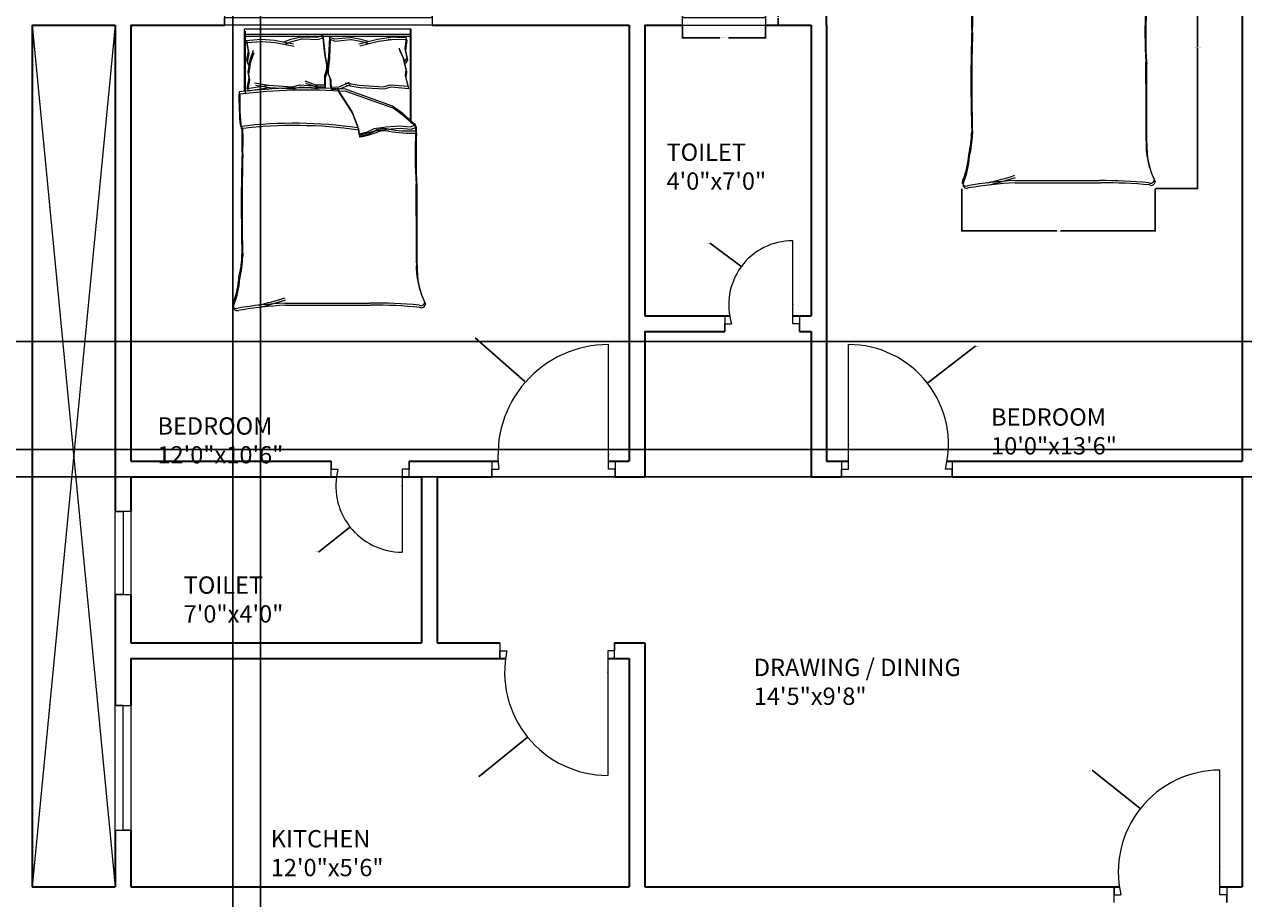
# Model space of a CAD drawing. Units: inches. Extents: x 1937 to 2996, y 1402 to 2323.
# Tile 7 of 10: x 2290 to 2643, y 1944 to 2197. Entities that reach past the tile are written whole.
import ezdxf

# ---------------------------------------------------------------- set-up
doc = ezdxf.new("R2010")
doc.units = ezdxf.units.IN
for name, color, linetype, lineweight in [('A-ANNO-DIMS', 2, 'Continuous', 18), ('A-AREA-IDEN', 7, 'Continuous', 18), ('A-DOOR', 11, 'Continuous', 18), ('A-FLOR-OPEN', 81, 'Continuous', 18), ('A-FURN', 8, 'Continuous', 13), ('A-GLAZ', 141, 'Continuous', 18), ('A-WALL', 7, 'Continuous', 35)]:
    doc.layers.add(name, color=color, linetype=linetype, lineweight=lineweight)
doc.styles.get("Standard").update_dxf_attribs({"font": 'arial.ttf'})
doc.dimstyles.get("Standard").update_dxf_attribs({"dimtxt": 0.18, "dimasz": 0.18, "dimexe": 0.18, "dimexo": 0.0625, "dimgap": 0.09, "dimtad": 0, "dimtih": 1, "dimtoh": 1, "dimdec": 4, "dimzin": 0, "dimdsep": 46, "dimtxsty": 'Standard', "dimcen": 0.09, "dimadec": 0, "dimazin": 0, "dimtfac": 1, "dimtdec": 4, "dimtofl": 0, "dimtmove": 0, "dimatfit": 3, "dimfxl": 1, "dimtolj": 1, "dimtzin": 0, "dimarcsym": 0})

# ---------------------------------------------------------------- blocks, each defined once
blk = doc.blocks.new('BED-DOUBLE')
for p, q in [((-24.01, -18.11), (-24.01, 0)), ((-24.01, -18.11), (-24.01, 0)), ((-24.01, 0), (24.01, 0)), ((23.78, 0), (23.78, -26.61)), ((23.78, 0), (23.78, -26.61)), ((24.01, 0), (24.01, -0.64)), ((-24.01, -1.53), (23.78, -1.53)), ((-24.01, -1.53), (23.78, -1.53)), ((-23.78, -18.75), (-23.78, -0.64)), ((-23.78, -18.75), (-23.78, -0.64)), ((-23.78, -2.17), (24.01, -2.17)), ((-23.78, -2.17), (24.01, -2.17)), ((-23.59, -3.34), (-19.3, -3.01)), ((-23.59, -3.34), (-19.31, -3.01)), ((-23.59, -3.32), (-23.01, -6.5)), ((-23.59, -3.32), (-23.01, -6.5)), ((-19.31, -3.01), (-19.2, -3.03)), ((-19.3, -3.01), (-19.2, -3.03)), ((-19.2, -3.03), (-15.38, -3.32)), ((-19.2, -3.03), (-15.38, -3.32)), ((-15.38, -3.32), (-9.88, -4.33)), ((-15.38, -3.32), (-9.88, -4.33)), ((-12.63, -3.75), (-10.61, -3.03)), ((-12.63, -3.75), (-10.61, -3.03)), ((-10.61, -3.03), (-7.71, -2.3)), ((-10.61, -3.03), (-7.71, -2.3)), ((-10.38, -3.67), (-7.49, -2.94)), ((-10.38, -3.67), (-7.49, -2.94)), ((-7.71, -2.3), (-7.39, -2.3)), ((-7.71, -2.3), (-7.39, -2.3)), ((-7.49, -2.94), (-7.16, -2.94)), ((-7.49, -2.94), (-7.16, -2.94)), ((-7.39, -2.3), (-2.95, -2.45)), ((-7.39, -2.3), (-2.95, -2.45)), ((-7.16, -2.94), (-2.72, -3.09)), ((-7.16, -2.94), (-2.72, -3.09)), ((-2.95, -2.45), (-1.5, -1.87)), ((-2.95, -2.45), (-1.5, -1.87)), ((-2.72, -3.09), (-1.27, -2.51)), ((-2.72, -3.09), (-1.27, -2.51)), ((-1.5, -1.87), (-0.92, -7.22)), ((-1.5, -1.87), (-0.92, -7.22)), ((-1.27, -2.51), (-0.7, -7.86)), ((-1.27, -2.51), (-0.7, -7.86)), ((0.49, -2.49), (0.25, -7.87)), ((0.49, -2.49), (0.25, -7.87)), ((0.72, -3.13), (0.48, -8.51)), ((0.72, -3.13), (0.48, -8.51)), ((1.97, -2.98), (0.49, -2.49)), ((1.97, -2.98), (0.49, -2.49)), ((2.2, -3.62), (0.72, -3.13)), ((2.2, -3.62), (0.72, -3.13)), ((6.4, -2.56), (1.97, -2.98)), ((6.4, -2.56), (1.97, -2.98)), ((6.63, -3.2), (2.2, -3.62)), ((6.63, -3.2), (2.2, -3.62)), ((6.72, -2.54), (6.4, -2.56)), ((6.72, -2.54), (6.4, -2.56)), ((6.95, -3.18), (6.63, -3.2)), ((6.95, -3.18), (6.63, -3.2)), ((9.65, -3.08), (6.72, -2.54)), ((9.65, -3.08), (6.72, -2.54)), ((9.88, -3.72), (6.95, -3.18)), ((9.88, -3.72), (6.95, -3.18)), ((14.43, -3.07), (9.01, -4.42)), ((14.43, -3.07), (9.01, -4.42)), ((11.72, -3.67), (9.65, -3.08)), ((11.72, -3.67), (9.65, -3.08)), ((18.23, -2.54), (14.43, -3.07)), ((18.23, -2.54), (14.43, -3.07)), ((18.46, -3.18), (14.66, -3.71)), ((18.46, -3.18), (14.66, -3.71)), ((22.63, -2.56), (17.23, -2.46)), ((17.23, -2.46), (18.23, -2.54)), ((22.63, -2.56), (17.23, -2.46)), ((17.23, -2.46), (18.23, -2.54)), ((22.86, -3.2), (17.45, -3.1)), ((17.45, -3.1), (18.46, -3.18)), ((22.86, -3.2), (17.45, -3.1)), ((17.45, -3.1), (18.46, -3.18)), ((22.63, -2.56), (22.25, -5.77)), ((22.63, -2.56), (22.25, -5.77)), ((22.86, -3.2), (22.48, -6.41)), ((22.86, -3.2), (22.48, -6.41)), ((24.01, -0.64), (24.01, -27.25)), ((24.01, -0.64), (24.01, -27.25)), ((-23.01, -6.5), (-23.45, -9.1)), ((-23.01, -6.5), (-23.45, -9.1)), ((-23.36, -3.98), (-19.08, -3.65)), ((-23.36, -3.98), (-19.08, -3.65)), ((-23.36, -3.96), (-22.78, -7.14)), ((-23.36, -3.96), (-22.78, -7.14)), ((-22.43, -8.96), (-21.42, -6.21)), ((-22.43, -8.96), (-21.42, -6.21)), ((-22.21, -9.59), (-21.19, -6.85)), ((-22.2, -9.59), (-21.19, -6.85)), ((-19.08, -3.65), (-18.97, -3.67)), ((-19.08, -3.65), (-18.97, -3.67)), ((-18.97, -3.67), (-15.15, -3.96)), ((-18.97, -3.67), (-15.15, -3.96)), ((-15.15, -3.96), (-9.65, -4.97)), ((-15.15, -3.96), (-9.65, -4.97)), ((-12.4, -4.39), (-10.38, -3.67)), ((-12.4, -4.39), (-10.38, -3.67)), ((14.66, -3.71), (9.24, -5.06)), ((14.66, -3.71), (9.24, -5.06)), ((11.94, -4.31), (9.88, -3.72)), ((11.94, -4.31), (9.88, -3.72)), ((21.83, -8.26), (20.64, -5.58)), ((21.82, -8.26), (20.64, -5.58)), ((22.05, -8.9), (20.87, -6.22)), ((22.05, -8.9), (20.87, -6.22)), ((22.25, -5.77), (22.84, -8.34)), ((22.25, -5.77), (22.84, -8.34)), ((22.48, -6.41), (23.07, -8.98)), ((22.48, -6.41), (23.07, -8.98)), ((-23.45, -9.1), (-22.87, -10.11)), ((-23.45, -9.1), (-22.87, -10.11)), ((-22.78, -7.14), (-23.22, -9.74)), ((-22.78, -7.14), (-23.22, -9.74)), ((-23.22, -9.74), (-22.64, -10.75)), ((-23.22, -9.74), (-22.64, -10.75)), ((-23.01, -12.57), (-22.43, -8.96)), ((-23.01, -12.57), (-22.43, -8.96)), ((-22.78, -13.21), (-22.2, -9.59)), ((-22.78, -13.21), (-22.21, -9.59)), ((-0.92, -7.22), (-0.35, -10.4)), ((-0.92, -7.22), (-0.35, -10.4)), ((-0.7, -7.86), (-0.12, -11.04)), ((-0.7, -7.86), (-0.12, -11.04)), ((-0.35, -10.4), (-0.35, -11.7)), ((-0.35, -10.4), (-0.35, -11.7)), ((0.25, -7.87), (-0.13, -11.08)), ((0.25, -7.87), (-0.13, -11.08)), ((0.48, -8.51), (0.1, -11.72)), ((0.48, -8.51), (0.1, -11.72)), ((22.63, -11.83), (21.82, -8.26)), ((22.63, -11.83), (21.83, -8.26)), ((22.86, -12.47), (22.05, -8.9)), ((22.86, -12.47), (22.05, -8.9)), ((22.84, -8.34), (22.33, -9.38)), ((22.84, -8.34), (22.33, -9.38)), ((23.07, -8.98), (22.56, -10.02)), ((23.07, -8.98), (22.56, -10.02)), ((-22.72, -14.16), (-23.01, -12.57)), ((-22.72, -14.16), (-23.01, -12.57)), ((-22.49, -14.8), (-22.78, -13.21)), ((-22.49, -14.8), (-22.78, -13.21)), ((-0.35, -11.7), (-0.92, -13.58)), ((-0.35, -11.7), (-0.92, -13.58)), ((-0.92, -13.58), (-0.92, -16.26)), ((-0.92, -13.58), (-0.92, -16.26)), ((-0.12, -12.34), (-0.7, -14.22)), ((-0.12, -12.34), (-0.7, -14.22)), ((-0.13, -11.08), (-0.05, -12.38)), ((-0.13, -11.08), (-0.05, -12.38)), ((-0.12, -11.04), (-0.12, -12.34)), ((-0.12, -11.04), (-0.12, -12.34)), ((-0.05, -12.38), (0.65, -14.22)), ((-0.05, -12.38), (0.65, -14.22)), ((0.1, -11.72), (0.18, -13.02)), ((0.1, -11.72), (0.18, -13.02)), ((0.18, -13.02), (0.87, -14.86)), ((0.18, -13.02), (0.87, -14.86)), ((22.44, -13.43), (22.63, -11.83)), ((22.44, -13.43), (22.63, -11.83)), ((23.21, -16.57), (22.44, -13.43)), ((23.21, -16.57), (22.44, -13.43)), ((22.67, -14.07), (22.86, -12.47)), ((22.67, -14.07), (22.86, -12.47)), ((23.44, -17.21), (22.67, -14.07)), ((23.44, -17.21), (22.67, -14.07)), ((-23.3, -17.34), (-22.72, -14.16)), ((-23.3, -17.34), (-22.72, -14.16)), ((-18.2, -16.62), (-23.3, -17.34)), ((-18.2, -16.62), (-23.3, -17.34)), ((-23.07, -17.98), (-22.49, -14.8)), ((-23.07, -17.98), (-22.49, -14.8)), ((-17.98, -17.26), (-23.07, -17.98)), ((-17.98, -17.26), (-23.07, -17.98)), ((-21.1, -15.63), (-17.07, -16.3)), ((-21.1, -15.63), (-17.07, -16.3)), ((-20.87, -16.27), (-16.84, -16.93)), ((-20.87, -16.27), (-16.84, -16.93)), ((-17.07, -16.3), (-18.2, -16.62)), ((-17.07, -16.3), (-18.2, -16.62)), ((-16.84, -16.93), (-17.98, -17.26)), ((-16.84, -16.93), (-17.98, -17.26)), ((-17.07, -16.3), (-10.06, -16.73)), ((-17.07, -16.3), (-10.06, -16.73)), ((-16.84, -16.93), (-9.83, -17.37)), ((-16.84, -16.93), (-9.83, -17.37)), ((-10.06, -16.73), (-8.1, -16.17)), ((-10.06, -16.73), (-8.1, -16.17)), ((-9.83, -17.37), (-7.87, -16.81)), ((-9.83, -17.37), (-7.87, -16.81)), ((-8.1, -16.17), (-2.97, -16.57)), ((-8.1, -16.17), (-2.97, -16.57)), ((-7.87, -16.81), (-2.74, -17.21)), ((-7.87, -16.81), (-2.74, -17.21)), ((-3.38, -16.26), (-6.53, -15.17)), ((-3.38, -16.26), (-6.53, -15.17)), ((-3.15, -16.9), (-6.3, -15.81)), ((-3.15, -16.9), (-6.3, -15.81)), ((-0.92, -16.26), (-3.38, -16.26)), ((-0.92, -16.26), (-3.38, -16.26)), ((-0.7, -16.9), (-3.15, -16.9)), ((-0.7, -16.9), (-3.15, -16.9)), ((-0.7, -14.22), (-0.7, -16.9)), ((-0.7, -14.22), (-0.7, -16.9)), ((0.65, -14.22), (0.81, -16.89)), ((0.65, -14.22), (0.81, -16.89)), ((0.81, -16.89), (3.27, -16.74)), ((0.81, -16.89), (3.27, -16.74)), ((0.87, -14.86), (1.04, -17.53)), ((0.87, -14.86), (1.04, -17.53)), ((1.04, -17.53), (3.49, -17.38)), ((1.04, -17.53), (3.49, -17.38)), ((2.77, -17.38), (6.97, -23.88)), ((2.77, -17.38), (6.96, -23.88)), ((3.27, -16.74), (6.34, -15.45)), ((3.27, -16.74), (6.34, -15.45)), ((3.49, -17.38), (6.56, -16.09)), ((3.49, -17.38), (6.56, -16.09)), ((13.16, -20.32), (4.82, -17.38)), ((13.16, -20.32), (4.82, -17.38)), ((5.08, -15.63), (9.11, -16.3)), ((5.08, -15.63), (9.11, -16.3)), ((5.31, -16.27), (9.34, -16.93)), ((5.31, -16.27), (9.34, -16.93)), ((9.11, -16.3), (16.12, -16.73)), ((9.11, -16.3), (16.12, -16.73)), ((9.34, -16.93), (16.35, -17.37)), ((9.34, -16.93), (16.35, -17.37)), ((16.12, -16.73), (18.08, -16.17)), ((16.12, -16.73), (18.08, -16.17)), ((16.35, -17.37), (18.31, -16.81)), ((16.35, -17.37), (18.31, -16.81)), ((18.08, -16.17), (23.21, -16.57)), ((18.08, -16.17), (23.21, -16.57)), ((18.31, -16.81), (23.44, -17.21)), ((18.31, -16.81), (23.44, -17.21)), ((3, -18.02), (7.19, -24.52)), ((3, -18.02), (7.19, -24.52)), ((13.39, -20.96), (5.05, -18.02)), ((13.39, -20.96), (5.05, -18.02)), ((18.74, -22.33), (13.16, -20.32)), ((18.74, -22.33), (13.16, -20.32)), ((18.96, -22.97), (13.39, -20.96)), ((18.96, -22.97), (13.39, -20.96)), ((6.96, -23.88), (8.67, -28.37)), ((6.97, -23.88), (8.67, -28.37)), ((7.19, -24.52), (8.9, -29)), ((7.19, -24.52), (8.9, -29)), ((21.68, -24.5), (18.74, -22.33)), ((21.68, -24.5), (18.74, -22.33)), ((21.91, -25.13), (18.96, -22.97)), ((21.91, -25.13), (18.96, -22.97)), ((25.38, -27.75), (21.68, -24.5)), ((25.38, -27.75), (21.68, -24.5)), ((16.88, -28.37), (20.75, -28.06)), ((16.88, -28.37), (20.75, -28.06)), ((20.75, -28.06), (23.85, -28.37)), ((20.75, -28.06), (23.85, -28.37)), ((25.61, -28.39), (21.91, -25.13)), ((25.61, -28.39), (21.91, -25.13)), ((23.85, -28.37), (25.38, -27.75)), ((23.85, -28.37), (25.38, -27.75)), ((25.46, -29.49), (25.38, -27.75, 3.87)), ((25.46, -29.49), (25.38, -27.75, 3.87)), ((8.67, -28.37), (8.98, -30.38)), ((8.67, -28.37), (8.98, -30.38)), ((8.9, -29), (9.21, -31.02)), ((8.9, -29), (9.21, -31.02)), ((8.98, -30.38), (11.46, -29.76)), ((8.98, -30.38), (11.46, -29.76)), ((9.21, -31.02), (11.68, -30.4)), ((9.21, -31.02), (11.68, -30.4)), ((11.46, -29.76), (13.47, -28.83)), ((11.46, -29.76), (13.47, -28.83)), ((11.68, -30.4), (13.7, -29.47)), ((11.68, -30.4), (13.7, -29.47)), ((13.47, -28.83), (16.88, -28.37)), ((13.47, -28.83), (16.88, -28.37)), ((13.7, -29.47), (17.11, -29)), ((13.7, -29.47), (17.1, -29)), ((17.1, -29), (20.98, -28.69)), ((17.11, -29), (20.98, -28.69)), ((20.98, -28.69), (24.07, -29)), ((20.98, -28.69), (24.07, -29)), ((24.07, -29), (25.61, -28.39)), ((24.07, -29), (25.61, -28.39)), ((25.69, -30.13), (25.61, -28.39, 3.87)), ((25.69, -30.13), (25.61, -28.39, 3.87)), ((-12.42, -79.25), (12.19, -79.25)), ((-12.42, -79.25), (12.19, -79.25)), ((-12.19, -79.88), (12.42, -79.88)), ((-12.19, -79.88), (12.42, -79.88))]:
    blk.add_line(p, q)
for centre, radius, start, end in [((-6.13, -182.05), 164.97, 86.0865, 96.7821), ((-6.13, -182.05), 164.97, 86.0865, 96.7821), ((57.68, -20.1), 83.31, 178.7218, 185.604), ((57.68, -20.1), 83.31, 178.7218, 185.604), ((57.91, -20.74), 83.31, 178.7218, 185.604), ((57.91, -20.74), 83.31, 178.7218, 185.604), ((-5.9, -182.69), 164.97, 86.0865, 96.7821), ((-5.9, -182.69), 164.97, 86.0865, 96.7821), ((-9.73, -156.32), 129.02, 81.7845, 96.9006), ((-9.73, -156.32), 129.02, 81.7845, 96.9006), ((-9.5, -156.96), 129.02, 81.7845, 96.9006), ((-9.5, -156.96), 129.02, 81.7845, 96.9006), ((-194.79, -31.17), 170.11, 358.4762, 1.0082), ((-194.79, -31.17), 170.11, 358.4762, 1.0082), ((-194.56, -31.81), 170.11, 358.4762, 1.0082), ((-194.56, -31.81), 170.11, 358.4762, 1.0082), ((9.15, -30.44), 0.185, 160.2464, 271.1377), ((9.15, -30.44), 0.185, 160.2464, 271.1377), ((3.67, -1.48), 29.65, 280.6617, 289.8806), ((3.67, -1.48), 29.65, 280.6617, 289.8806), ((9.38, -31.08), 0.185, 160.2464, 271.1377), ((9.38, -31.08), 0.185, 160.2464, 271.1377), ((3.9, -2.12), 29.65, 280.6617, 289.8806), ((3.9, -2.12), 29.65, 280.6617, 289.8806), ((16.26, -35.07), 6.22, 78.6608, 113.7384), ((16.26, -35.07), 6.22, 78.6608, 113.7384), ((16.49, -35.71), 6.22, 78.6608, 113.7384), ((16.49, -35.71), 6.22, 78.6608, 113.7384), ((23.84, 6.66), 36.18, 259.8763, 272.5657), ((23.84, 6.66), 36.18, 259.8763, 272.5657), ((24.07, 6.02), 36.18, 259.8763, 272.5657), ((24.07, 6.02), 36.18, 259.8763, 272.5657), ((154.78, -36.32), 129.5, 176.9791, 183.8365), ((154.78, -36.32), 129.5, 176.9791, 183.8365), ((155.01, -36.95), 129.5, 176.9791, 183.8365), ((155.01, -36.95), 129.5, 176.9791, 183.8365), ((457.34, -50.61), 482.31, 178.2277, 181.7185), ((457.34, -50.61), 482.31, 178.2277, 181.7185), ((457.57, -51.25), 482.31, 178.2277, 181.7185), ((457.57, -51.25), 482.31, 178.2277, 181.7185), ((-4536.23, -67.82), 4561.86, 0.00217, 0.28689), ((-4536.23, -67.82), 4561.86, 0.00217, 0.28689), ((-4536, -68.46), 4561.86, 0.00217, 0.28689), ((-4536, -68.46), 4561.86, 0.00217, 0.28689), ((-54.38, -64.52), 29.63, 346.0648, 358.9113), ((-54.38, -64.52), 29.63, 346.0648, 358.9113), ((-54.16, -65.15), 29.63, 346.0648, 358.9113), ((-54.16, -65.15), 29.63, 346.0648, 358.9113), ((48.67, -68.67), 23.07, 177.4714, 206.4681), ((48.67, -68.67), 23.07, 177.4714, 206.4681), ((48.9, -69.31), 23.07, 177.4714, 206.4681), ((48.9, -69.31), 23.07, 177.4714, 206.4681), ((-49.14, -70.28), 23.56, 337.9751, 356.652), ((-49.14, -70.28), 23.56, 337.9751, 356.652), ((-48.92, -70.91), 23.56, 337.9751, 356.652), ((-48.92, -70.91), 23.56, 337.9751, 356.652), ((-26.4, -79.72), 1.09, 146.1736, 293.4781), ((-26.4, -79.72), 1.09, 146.1736, 293.4781), ((-26.17, -80.36), 1.09, 146.1736, 293.4781), ((-26.17, -80.36), 1.09, 146.1736, 293.4781), ((-6.06, -200.84), 121.76, 92.9958, 99.4091), ((-6.06, -200.84), 121.76, 92.9958, 99.4091), ((-5.83, -201.48), 121.76, 92.9958, 99.4091), ((-5.83, -201.48), 121.76, 92.9958, 99.4091), ((-44.71, 23.71), 106.46, 283.3832, 287.7053), ((-44.71, 23.71), 106.46, 283.3832, 287.7053), ((-44.48, 23.07), 106.46, 283.3832, 287.7053), ((-44.48, 23.07), 106.46, 283.3832, 287.7053), ((13.67, -212.28), 133.04, 84.4998, 90.6351), ((13.67, -212.28), 133.04, 84.4998, 90.6351), ((13.9, -212.92), 133.04, 84.4998, 90.6351), ((13.9, -212.92), 133.04, 84.4998, 90.6351), ((26.93, -78.87), 1.1, 242.6588, 356.02), ((26.93, -78.87), 1.1, 242.6588, 356.02), ((27.15, -79.51), 1.1, 242.6588, 356.02), ((27.15, -79.51), 1.1, 242.6588, 356.02)]:
    blk.add_arc(centre, radius, start, end)
blk = doc.blocks.new('WINDOW-60IN')
for p, q in [((0, 2.25), (0, -2.25)), ((0, 2.25), (60, 2.25)), ((0, -2.25), (0, 0)), ((0, 0), (60, 0)), ((60, 0), (60, 2.25)), ((60, 2.25), (60, -2.25)), ((60, -2.25), (0, -2.25))]:
    blk.add_line(p, q)
blk = doc.blocks.new('WINDOW-36IN')
for p, q in [((0, 2.25), (0, -2.25)), ((0, 2.25), (36, 2.25)), ((36, 0), (36, 2.25)), ((36, 2.25), (36, -2.25)), ((0, -2.25), (0, 0)), ((0, 0), (36, 0)), ((36, -2.25), (0, -2.25))]:
    blk.add_line(p, q)
blk = doc.blocks.new('WINDOW-24IN-JAMB-B')
for p, q in [((0, -2.25), (0, 2.25)), ((0, 2.25), (0, 0)), ((24, 2.25), (0, 2.25)), ((0, 0), (24, 0)), ((24, 0), (24, 2.25)), ((24, 2.25), (24, -2.25)), ((0, -2.25), (24, -2.25))]:
    blk.add_line(p, q)
blk = doc.blocks.new('VOID-MARK-24X249')
for p, q in [((24, 249), (0, 0)), ((0, 249), (24, 0))]:
    blk.add_line(p, q)
blk = doc.blocks.new('*D9')
at = {"layer": 'A-ANNO-DIMS', "color": 0, "lineweight": -2, "transparency": 16777216}
for p, q in [((2617.12, 2230.66), (2629.47, 2230.66)), ((2629.29, 2230.48), (2629.29, 2190.07)), ((2629.29, 2149.29), (2629.29, 2189.7)), ((2617.12, 2149.11), (2629.47, 2149.11))]:
    blk.add_line(p, q, dxfattribs=at)
at = {"layer": 'A-ANNO-DIMS', "color": 0, "transparency": 16777216}
for points in [[(2629.26, 2230.48), (2629.32, 2230.48), (2629.29, 2230.66)], [(2629.26, 2149.29), (2629.32, 2149.29), (2629.29, 2149.11)]]:
    blk.add_solid(points, dxfattribs=at)
at = {"layer": 'Defpoints', "color": 0, "transparency": 16777216}
for p in [(2617.06, 2230.66), (2629.29, 2230.66), (2617.06, 2149.11)]:
    blk.add_point(p, dxfattribs=at)
at = {"layer": 'A-ANNO-DIMS', "color": 0, "transparency": 16777216, "insert": (2629.29, 2189.88), "char_height": 0.18, "attachment_point": 5}
blk.add_mtext('\\A1;DOUBLE BED 82 TYP.', dxfattribs=at)
blk = doc.blocks.new('*D10')
at = {"layer": 'A-ANNO-DIMS', "color": 0, "lineweight": -2, "transparency": 16777216}
for p, q in [((2561.23, 2149.05), (2561.23, 2136.7)), ((2617.06, 2149.05), (2617.06, 2136.7)), ((2561.41, 2136.88), (2588.62, 2136.88)), ((2616.88, 2136.88), (2589.67, 2136.88))]:
    blk.add_line(p, q, dxfattribs=at)
at = {"layer": 'A-ANNO-DIMS', "color": 0, "transparency": 16777216}
for points in [[(2561.41, 2136.91), (2561.41, 2136.85), (2561.23, 2136.88)], [(2616.88, 2136.91), (2616.88, 2136.85), (2617.06, 2136.88)]]:
    blk.add_solid(points, dxfattribs=at)
at = {"layer": 'Defpoints', "color": 0, "transparency": 16777216}
for p in [(2561.23, 2149.11), (2617.06, 2149.11), (2617.06, 2136.88)]:
    blk.add_point(p, dxfattribs=at)
at = {"layer": 'A-ANNO-DIMS', "color": 0, "transparency": 16777216, "insert": (2589.14, 2136.88), "char_height": 0.18, "attachment_point": 5}
blk.add_mtext('\\A1;56 TYP.', dxfattribs=at)
blk = doc.blocks.new('*D17')
at = {"layer": 'A-ANNO-DIMS', "color": 0, "lineweight": -2, "transparency": 16777216}
for p, q in [((2480.52, 2196.24), (2480.52, 2192.53)), ((2504.52, 2196.24), (2504.52, 2192.53)), ((2480.7, 2192.71), (2491.28, 2192.71)), ((2504.34, 2192.71), (2493.75, 2192.71))]:
    blk.add_line(p, q, dxfattribs=at)
at = {"layer": 'A-ANNO-DIMS', "color": 0, "transparency": 16777216}
for points in [[(2480.7, 2192.74), (2480.7, 2192.68), (2480.52, 2192.71)], [(2504.34, 2192.74), (2504.34, 2192.68), (2504.52, 2192.71)]]:
    blk.add_solid(points, dxfattribs=at)
at = {"layer": 'Defpoints', "color": 0, "transparency": 16777216}
for p in [(2480.52, 2196.31), (2504.52, 2196.31), (2504.52, 2192.71)]:
    blk.add_point(p, dxfattribs=at)
at = {"layer": 'A-ANNO-DIMS', "color": 0, "transparency": 16777216, "insert": (2492.52, 2192.71), "char_height": 0.18, "attachment_point": 5}
blk.add_mtext('\\A1;WINDOW B 24 TYP.', dxfattribs=at)
blk = doc.blocks.new('*D18')
at = {"layer": 'A-ANNO-DIMS', "color": 0, "lineweight": -2, "transparency": 16777216}
for p, q in [((2504.58, 2200.81), (2508.3, 2200.81)), ((2508.12, 2200.63), (2508.12, 2198.74)), ((2508.12, 2196.49), (2508.12, 2198.37)), ((2504.58, 2196.31), (2508.3, 2196.31))]:
    blk.add_line(p, q, dxfattribs=at)
at = {"layer": 'A-ANNO-DIMS', "color": 0, "transparency": 16777216}
for points in [[(2508.09, 2200.63), (2508.15, 2200.63), (2508.12, 2200.81)], [(2508.09, 2196.49), (2508.15, 2196.49), (2508.12, 2196.31)]]:
    blk.add_solid(points, dxfattribs=at)
at = {"layer": 'Defpoints', "color": 0, "transparency": 16777216}
for p in [(2504.52, 2200.81), (2508.12, 2200.81), (2504.52, 2196.31)]:
    blk.add_point(p, dxfattribs=at)
at = {"layer": 'A-ANNO-DIMS', "color": 0, "transparency": 16777216, "insert": (2508.12, 2198.56), "char_height": 0.18, "attachment_point": 5}
blk.add_mtext('\\A1;5 TYP.', dxfattribs=at)
blk = doc.blocks.new('*D36')
at = {"layer": 'A-ANNO-DIMS', "color": 0, "lineweight": -2, "transparency": 16777216}
for p, q in [((2350.61, 1896.12), (2350.61, 2283.14)), ((2350.79, 2282.96), (2354.46, 2282.96)), ((2358.43, 2282.96), (2354.76, 2282.96)), ((2358.61, 1896.12), (2358.61, 2283.14))]:
    blk.add_line(p, q, dxfattribs=at)
at = {"layer": 'A-ANNO-DIMS', "color": 0, "transparency": 16777216}
for points in [[(2350.79, 2282.99), (2350.79, 2282.93), (2350.61, 2282.96)], [(2358.43, 2282.99), (2358.43, 2282.93), (2358.61, 2282.96)]]:
    blk.add_solid(points, dxfattribs=at)
at = {"layer": 'Defpoints', "color": 0, "transparency": 16777216}
for p in [(2358.61, 2282.96), (2350.61, 1896.06), (2358.61, 1896.06)]:
    blk.add_point(p, dxfattribs=at)
at = {"layer": 'A-ANNO-DIMS', "color": 0, "transparency": 16777216, "insert": (2354.61, 2282.96), "char_height": 0.18, "attachment_point": 5}
blk.add_mtext('\\A1;8', dxfattribs=at)
blk = doc.blocks.new('*D51')
at = {"layer": 'A-ANNO-DIMS', "color": 0, "lineweight": -2, "transparency": 16777216}
for p, q in [((2175.71, 2073.74), (2970.48, 2073.74)), ((2970.3, 2073.56), (2970.3, 2069.95)), ((2970.3, 2065.99), (2970.3, 2069.59)), ((2175.71, 2065.81), (2970.48, 2065.81))]:
    blk.add_line(p, q, dxfattribs=at)
at = {"layer": 'A-ANNO-DIMS', "color": 0, "transparency": 16777216}
for points in [[(2970.27, 2073.56), (2970.33, 2073.56), (2970.3, 2073.74)], [(2970.27, 2065.99), (2970.33, 2065.99), (2970.3, 2065.81)]]:
    blk.add_solid(points, dxfattribs=at)
at = {"layer": 'Defpoints', "color": 0, "transparency": 16777216}
for p in [(2175.65, 2073.74), (2970.3, 2073.74), (2175.65, 2065.81)]:
    blk.add_point(p, dxfattribs=at)
at = {"layer": 'A-ANNO-DIMS', "color": 0, "transparency": 16777216, "insert": (2970.3, 2069.77), "char_height": 0.18, "attachment_point": 5}
blk.add_mtext('\\A1;7.931', dxfattribs=at)
blk = doc.blocks.new('*D52')
at = {"layer": 'A-ANNO-DIMS', "color": 0, "lineweight": -2, "transparency": 16777216}
for p, q in [((2175.71, 2104.94), (2970.48, 2104.94)), ((2970.3, 2104.76), (2970.3, 2089.52)), ((2970.3, 2073.92), (2970.3, 2089.16)), ((2175.71, 2073.74), (2970.48, 2073.74))]:
    blk.add_line(p, q, dxfattribs=at)
at = {"layer": 'A-ANNO-DIMS', "color": 0, "transparency": 16777216}
for points in [[(2970.27, 2104.76), (2970.33, 2104.76), (2970.3, 2104.94)], [(2970.27, 2073.92), (2970.33, 2073.92), (2970.3, 2073.74)]]:
    blk.add_solid(points, dxfattribs=at)
at = {"layer": 'Defpoints', "color": 0, "transparency": 16777216}
for p in [(2175.65, 2104.94), (2970.3, 2104.94), (2175.65, 2073.74)]:
    blk.add_point(p, dxfattribs=at)
at = {"layer": 'A-ANNO-DIMS', "color": 0, "transparency": 16777216, "insert": (2970.3, 2089.34), "char_height": 0.18, "attachment_point": 5}
blk.add_mtext('\\A1;31.204', dxfattribs=at)
blk = doc.blocks.new('*D55')
at = {"layer": 'A-ANNO-DIMS', "color": 0, "lineweight": -2, "transparency": 16777216}
for p, q in [((2420.58, 2105.85), (2420.76, 2105.85)), ((2420.76, 2105.85), (2435, 2093.33)), ((2459.01, 2072.16), (2459.19, 2072.16)), ((2459.1, 2072.07), (2459.1, 2072.25))]:
    blk.add_line(p, q, dxfattribs=at)
at = {"layer": 'A-ANNO-DIMS', "color": 0, "transparency": 16777216}
blk.add_solid([(2435.02, 2093.35), (2434.98, 2093.31), (2435.13, 2093.21)], dxfattribs=at)
at = {"layer": 'Defpoints', "color": 0, "transparency": 16777216}
for p in [(2435.13, 2093.21), (2459.1, 2072.16)]:
    blk.add_point(p, dxfattribs=at)
at = {"layer": 'A-ANNO-DIMS', "color": 0, "transparency": 16777216, "insert": (2420.17, 2105.85), "char_height": 0.18, "attachment_point": 5}
blk.add_mtext('\\A1;R31.9', dxfattribs=at)
blk = doc.blocks.new('*D57')
at = {"layer": 'A-ANNO-DIMS', "color": 0, "lineweight": -2, "transparency": 16777216}
for p, q in [((2458.82, 2009.36), (2459, 2009.36)), ((2458.91, 2009.27), (2458.91, 2009.45)), ((2421.86, 1979.35), (2435.61, 1990.49)), ((2421.68, 1979.35), (2421.86, 1979.35))]:
    blk.add_line(p, q, dxfattribs=at)
at = {"layer": 'A-ANNO-DIMS', "color": 0, "transparency": 16777216}
blk.add_solid([(2435.59, 1990.51), (2435.63, 1990.47), (2435.75, 1990.6)], dxfattribs=at)
at = {"layer": 'Defpoints', "color": 0, "transparency": 16777216}
for p in [(2458.91, 2009.36), (2435.75, 1990.6)]:
    blk.add_point(p, dxfattribs=at)
at = {"layer": 'A-ANNO-DIMS', "color": 0, "transparency": 16777216, "insert": (2421.27, 1979.35), "char_height": 0.18, "attachment_point": 5}
blk.add_mtext('\\A1;R29.8', dxfattribs=at)
blk = doc.blocks.new('*D59')
at = {"layer": 'A-ANNO-DIMS', "color": 0, "lineweight": -2, "transparency": 16777216}
for p, q in [((2598.81, 1980.92), (2598.99, 1980.92)), ((2598.99, 1980.92), (2612.64, 1970.07)), ((2635.68, 1951.69), (2635.86, 1951.69)), ((2635.77, 1951.6), (2635.77, 1951.78))]:
    blk.add_line(p, q, dxfattribs=at)
at = {"layer": 'A-ANNO-DIMS', "color": 0, "transparency": 16777216}
blk.add_solid([(2612.66, 1970.1), (2612.62, 1970.05), (2612.78, 1969.96)], dxfattribs=at)
at = {"layer": 'Defpoints', "color": 0, "transparency": 16777216}
for p in [(2612.78, 1969.96), (2635.77, 1951.69)]:
    blk.add_point(p, dxfattribs=at)
at = {"layer": 'A-ANNO-DIMS', "color": 0, "transparency": 16777216, "insert": (2598.33, 1980.92), "char_height": 0.18, "attachment_point": 5}
blk.add_mtext('\\A1;R29.37', dxfattribs=at)
blk = doc.blocks.new('*D63')
at = {"layer": 'A-ANNO-DIMS', "color": 0, "lineweight": -2, "transparency": 16777216}
for p, q in [((2564.94, 2103.53), (2551.4, 2093.01)), ((2565.12, 2103.53), (2564.94, 2103.53)), ((2528.37, 2075.18), (2528.55, 2075.18)), ((2528.46, 2075.09), (2528.46, 2075.27))]:
    blk.add_line(p, q, dxfattribs=at)
at = {"layer": 'A-ANNO-DIMS', "color": 0, "transparency": 16777216}
blk.add_solid([(2551.39, 2093.04), (2551.42, 2092.99), (2551.26, 2092.9)], dxfattribs=at)
at = {"layer": 'Defpoints', "color": 0, "transparency": 16777216}
for p in [(2551.26, 2092.9), (2528.46, 2075.18)]:
    blk.add_point(p, dxfattribs=at)
at = {"layer": 'A-ANNO-DIMS', "color": 0, "transparency": 16777216, "insert": (2565.67, 2103.53), "char_height": 0.18, "attachment_point": 5}
blk.add_mtext('\\A1;R28.874', dxfattribs=at)
blk = doc.blocks.new('*D76')
at = {"layer": 'A-ANNO-DIMS', "color": 0, "lineweight": -2, "transparency": 16777216}
for p, q in [((2399.43, 2063.21), (2399.61, 2063.21)), ((2399.52, 2063.12), (2399.52, 2063.3)), ((2375.5, 2044.17), (2384.36, 2051.2)), ((2375.32, 2044.17), (2375.5, 2044.17))]:
    blk.add_line(p, q, dxfattribs=at)
at = {"layer": 'A-ANNO-DIMS', "color": 0, "transparency": 16777216}
blk.add_solid([(2384.34, 2051.23), (2384.38, 2051.18), (2384.5, 2051.31)], dxfattribs=at)
at = {"layer": 'Defpoints', "color": 0, "transparency": 16777216}
for p in [(2399.52, 2063.21), (2384.5, 2051.31)]:
    blk.add_point(p, dxfattribs=at)
at = {"layer": 'A-ANNO-DIMS', "color": 0, "transparency": 16777216, "insert": (2374.77, 2044.17), "char_height": 0.18, "attachment_point": 5}
blk.add_mtext('\\A1;R19.158', dxfattribs=at)
blk = doc.blocks.new('*D77')
at = {"layer": 'A-ANNO-DIMS', "color": 0, "lineweight": -2, "transparency": 16777216}
for p, q in [((2488.45, 2133.24), (2488.63, 2133.24)), ((2488.63, 2133.24), (2497.37, 2126.72)), ((2512.25, 2115.58), (2512.43, 2115.58)), ((2512.34, 2115.49), (2512.34, 2115.67))]:
    blk.add_line(p, q, dxfattribs=at)
at = {"layer": 'A-ANNO-DIMS', "color": 0, "transparency": 16777216}
blk.add_solid([(2497.39, 2126.75), (2497.36, 2126.7), (2497.52, 2126.61)], dxfattribs=at)
at = {"layer": 'Defpoints', "color": 0, "transparency": 16777216}
for p in [(2497.52, 2126.61), (2512.34, 2115.58)]:
    blk.add_point(p, dxfattribs=at)
at = {"layer": 'A-ANNO-DIMS', "color": 0, "transparency": 16777216, "insert": (2487.97, 2133.24), "char_height": 0.18, "attachment_point": 5}
blk.add_mtext('\\A1;R18.48', dxfattribs=at)

msp = doc.modelspace()

# ---------------------------------------------------------------- linework, layer by layer
at = {"layer": 'A-DOOR'}
for p, q in [((2512.3375, 2110.0561), (2512.3375, 2134.0561)), ((2492.7032, 2112.3061), (2492.7032, 2107.8061)), ((2492.7032, 2107.8061), (2492.7032, 2110.0561)), ((2492.7032, 2110.0561), (2494.7032, 2110.0561)), ((2514.3375, 2110.0561), (2512.3375, 2110.0561)), ((2514.3375, 2112.3061), (2514.3375, 2107.8061)), ((2514.3375, 2107.8061), (2514.3375, 2110.0561)), ((2459.0977, 2068.0561), (2459.0977, 2104.0561)), ((2528.4647, 2068.0561), (2528.4647, 2104.0561)), ((2378.9808, 2065.8061), (2378.9808, 2070.3061)), ((2378.9808, 2070.3061), (2378.9808, 2068.0561)), ((2378.9808, 2068.0561), (2380.9808, 2068.0561)), ((2401.5169, 2068.0561), (2399.5169, 2068.0561)), ((2399.5169, 2068.0561), (2399.5169, 2044.0561)), ((2401.5169, 2065.8061), (2401.5169, 2070.3061)), ((2401.5169, 2070.3061), (2401.5169, 2068.0561)), ((2425.4624, 2070.3061), (2425.4624, 2065.8061)), ((2425.4624, 2065.8061), (2425.4624, 2068.0561)), ((2425.4624, 2068.0561), (2427.4624, 2068.0561)), ((2461.0977, 2068.0561), (2459.0977, 2068.0561)), ((2461.0977, 2070.3061), (2461.0977, 2065.8061)), ((2461.0977, 2065.8061), (2461.0977, 2068.0561)), ((2526.4647, 2070.3061), (2526.4647, 2065.8061)), ((2526.4647, 2065.8061), (2526.4647, 2068.0561)), ((2526.4647, 2068.0561), (2528.4647, 2068.0561)), ((2558.4451, 2068.0561), (2556.4451, 2068.0561)), ((2558.4451, 2070.3061), (2558.4451, 2065.8061)), ((2558.4451, 2065.8061), (2558.4451, 2068.0561)), ((2427.765, 2017.8061), (2427.765, 2013.3061)), ((2427.765, 2013.3061), (2427.765, 2015.5561)), ((2427.765, 2015.5561), (2429.765, 2015.5561)), ((2460.9117, 2015.5561), (2458.9117, 2015.5561)), ((2458.9117, 2015.5561), (2458.9117, 1979.5561)), ((2460.9117, 2013.3061), (2460.9117, 2017.8061)), ((2460.9117, 2017.8061), (2460.9117, 2015.5561)), ((2635.7727, 1945.0561), (2635.7727, 1981.0561)), ((2605.163, 1942.8061), (2605.163, 1947.3061)), ((2605.163, 1947.3061), (2605.163, 1945.0561)), ((2605.163, 1945.0561), (2607.163, 1945.0561)), ((2637.7727, 1945.0561), (2635.7727, 1945.0561)), ((2637.7727, 1947.3061), (2637.7727, 1942.8061)), ((2637.7727, 1942.8061), (2637.7727, 1945.0561))]:
    msp.add_line(p, q, dxfattribs=at)
for centre, radius, start, end in [((2512.3375, 2115.5776), 18.4786, 90, 197.385677), ((2459.0977, 2072.1563), 31.8999, 90, 187.384751), ((2528.4647, 2075.1825), 28.8736, 345.71095, 90), ((2399.5169, 2063.2142), 19.1581, 165.360552, 270), ((2458.9117, 2009.3551), 29.799, 167.989364, 270), ((2635.7727, 1951.6879), 29.3683, 90, 193.050702)]:
    msp.add_arc(centre, radius, start, end, dxfattribs=at)
at = {"layer": 'A-GLAZ'}
for p, q in [((2321.1473, 2055.8311), (2316.6473, 2055.8311)), ((2316.6473, 2055.8311), (2318.8973, 2055.8311)), ((2316.6473, 2031.8311), (2316.6473, 2055.6277)), ((2318.8973, 2055.8311), (2318.8973, 2031.8311)), ((2321.1473, 2055.8311), (2321.1473, 2031.8311)), ((2318.8973, 2031.8311), (2316.6473, 2031.8311)), ((2316.6473, 2031.8311), (2321.1473, 2031.8311))]:
    msp.add_line(p, q, dxfattribs=at)
at = {"layer": 'A-WALL'}
for p, q in [((2642.1473, 2232.3061), (2642.1473, 2070.3061)), ((2522.1473, 2196.3061), (2522.1473, 2200.8061)), ((2292.6473, 2196.3061), (2292.6473, 1947.3061)), ((2292.6473, 2196.3061), (2316.6473, 2196.3061)), ((2316.6473, 2196.3061), (2316.6473, 2055.8311)), ((2321.1473, 2196.3061), (2321.1473, 2070.3061)), ((2321.1473, 2196.3061), (2348.1952, 2196.3061)), ((2408.1952, 2196.3061), (2465.1473, 2196.3061)), ((2465.1473, 2196.3061), (2465.1473, 2070.3061)), ((2469.6473, 2196.3061), (2469.6473, 2112.3061)), ((2469.6473, 2196.3061), (2480.5154, 2196.3061)), ((2504.5154, 2196.3061), (2517.6473, 2196.3061)), ((2517.6473, 2196.3061), (2517.6473, 2112.3061)), ((2522.1473, 2196.3061), (2522.1473, 2070.3061)), ((2469.6473, 2112.3061), (2494.1509, 2112.3061)), ((2512.3375, 2112.3061), (2517.6473, 2112.3061)), ((2469.6473, 2107.8061), (2492.7032, 2107.8061)), ((2469.6473, 2107.8061), (2469.6473, 2065.8061)), ((2514.3375, 2107.8061), (2517.6473, 2107.8061)), ((2517.6473, 2107.8061), (2517.6473, 2065.8061)), ((2321.1473, 2070.3061), (2378.9808, 2070.3061)), ((2401.5169, 2070.3061), (2427.2515, 2070.3061)), ((2459.0977, 2070.3061), (2465.1473, 2070.3061)), ((2522.1473, 2070.3061), (2528.4647, 2070.3061)), ((2556.9236, 2070.3061), (2642.1473, 2070.3061)), ((2321.1473, 2065.8061), (2380.5349, 2065.8061)), ((2321.1473, 2065.8061), (2321.1473, 2055.8311)), ((2399.5169, 2065.8061), (2405.1473, 2065.8061)), ((2405.1473, 2065.8061), (2405.1473, 2017.8061)), ((2409.6473, 2065.8061), (2409.6473, 2017.8061)), ((2409.6473, 2065.8061), (2425.4624, 2065.8061)), ((2461.0977, 2065.8061), (2469.6473, 2065.8061)), ((2517.6473, 2065.8061), (2526.4647, 2065.8061)), ((2558.4451, 2065.8061), (2642.1473, 2065.8061)), ((2642.1473, 2065.8061), (2642.1473, 1947.3061)), ((2316.6473, 2031.8311), (2316.6473, 1999.753)), ((2321.1473, 2031.8311), (2321.1473, 2017.8061)), ((2321.1473, 2017.8061), (2405.1473, 2017.8061)), ((2409.6473, 2017.8061), (2427.765, 2017.8061)), ((2460.9117, 2017.8061), (2469.6473, 2017.8061)), ((2469.6473, 2017.8061), (2469.6473, 1947.3061)), ((2321.1473, 2013.3061), (2429.3757, 2013.3061)), ((2321.1473, 2013.3061), (2321.1473, 1999.753)), ((2458.9117, 2013.3061), (2465.1473, 2013.3061)), ((2465.1473, 2013.3061), (2465.1473, 1947.3061)), ((2316.6473, 1963.753), (2316.6473, 1947.3061)), ((2321.1473, 1963.753), (2321.1473, 1947.3061)), ((2292.6473, 1947.3061), (2316.6473, 1947.3061)), ((2321.1473, 1947.3061), (2465.1473, 1947.3061)), ((2469.6473, 1947.3061), (2606.7331, 1947.3061)), ((2635.7727, 1947.3061), (2642.1473, 1947.3061))]:
    msp.add_line(p, q, dxfattribs=at)

# ---------------------------------------------------------------- block references
at = {"layer": 'A-FLOR-OPEN'}
msp.add_blockref('VOID-MARK-24X249', (2292.6473, 1947.3061), dxfattribs=at)
at = {"layer": 'A-FURN'}
for p in [(2588.8017, 2230.6586), (2378.0114, 2195.2884)]:
    msp.add_blockref('BED-DOUBLE', p, dxfattribs=at)
at = {"layer": 'A-GLAZ'}
for name, p in [('WINDOW-60IN', (2348.1952, 2198.5561)), ('WINDOW-24IN-JAMB-B', (2480.5154, 2198.5561))]:
    msp.add_blockref(name, p, dxfattribs=at)
at = {"layer": 'A-GLAZ', "rotation": 90}
msp.add_blockref('WINDOW-36IN', (2318.8973, 1963.753), dxfattribs=at)

# ---------------------------------------------------------------- texts
at = {"layer": 'A-AREA-IDEN', "char_height": 5, "attachment_point": 1}
for s, width, insert in [('TOILET\\P4\'0"x7\'0"', 94.588971, (2475.8836, 2162.1275)), ('BEDROOM\\P10\'0"x13\'6"', 122.824616, (2569.6426, 2085.612)), ('BEDROOM\\P12\'0"x10\'6"', 109.140116, (2328.8371, 2083.0158)), ('TOILET\\P7\'0"x4\'0"', 110.63972, (2336.4104, 2037.0384)), ('DRAWING / DINING\\P14\'5"x9\'8"', 212.274887, (2501.0972, 2013.2582)), ('KITCHEN\\P12\'0"x5\'6"', 217.221468, (2361.5689, 1963.7359))]:
    msp.add_mtext_dynamic_manual_height_columns(s, width=width, gutter_width=12.5, heights=[0], dxfattribs=dict(at, insert=insert))

# ---------------------------------------------------------------- dimensions: what is measured, and where the dimension line sits
at = {"layer": 'A-ANNO-DIMS'}
dim = msp.add_linear_dim(base=(2358.6104, 2282.9561), p1=(2350.6104, 1896.0561), p2=(2358.6104, 1896.0561), dimstyle='Standard', override={"dimdec": 0, "dimlfac": 1, "dimrnd": 0, "dimzin": 0, "dimdsep": 46, "dimlunit": 2}, dxfattribs=at)
dim.commit()
dim.dimension.update_dxf_attribs({"geometry": '*D36', "text_midpoint": (2354.6104, 2282.9561)})
for base, p1, p2, text, picture, middle in [((2629.2877, 2230.6586), (2617.0554, 2149.11), (2617.0554, 2230.6586), 'DOUBLE BED <> TYP.', '*D9', (2629.2877, 2189.8843)), ((2508.1154072539, 2200.8061190364), (2504.5154072539, 2196.3061190364), (2504.5154072539, 2200.8061190364), '<> TYP.', '*D18', (2508.1154072539, 2198.5561190364))]:
    dim = msp.add_linear_dim(base=base, p1=p1, p2=p2, angle=90, text=text, dimstyle='Standard', override={"dimdec": 0, "dimlfac": 1, "dimrnd": 0, "dimzin": 0, "dimdsep": 46, "dimlunit": 2}, dxfattribs=at)
    dim.commit()
    dim.dimension.update_dxf_attribs({"geometry": picture, "text_midpoint": middle})
for base, p1, p2, text, picture, middle in [((2504.5154, 2192.7061), (2480.5154, 2196.3061), (2504.5154, 2196.3061), 'WINDOW B <> TYP.', '*D17', (2492.5154, 2192.7061)), ((2617.0554, 2136.8777), (2561.2309, 2149.11), (2617.0554, 2149.11), '<> TYP.', '*D10', (2589.1431, 2136.8777))]:
    dim = msp.add_linear_dim(base=base, p1=p1, p2=p2, text=text, dimstyle='Standard', override={"dimdec": 0, "dimlfac": 1, "dimrnd": 0, "dimzin": 0, "dimdsep": 46, "dimlunit": 2}, dxfattribs=at)
    dim.commit()
    dim.dimension.update_dxf_attribs({"geometry": picture, "text_midpoint": middle})
for center, mpoint, override, picture, middle in [((2512.3375, 2115.5776), (2497.5173, 2126.6147), {"dimdec": 2, "dimlfac": 1, "dimrnd": 0, "dimzin": 0, "dimdsep": 46, "dimlunit": 2}, '*D77', (2487.9652, 2133.237)), ((2459.0977, 2072.1563), (2435.1349, 2093.2131), {"dimdec": 1, "dimlfac": 1, "dimrnd": 0, "dimzin": 0, "dimdsep": 46, "dimlunit": 2}, '*D55', (2420.1672, 2105.8471)), ((2528.4647, 2075.1825), (2551.2623, 2092.9013), {"dimdec": 3, "dimlfac": 1, "dimrnd": 0, "dimzin": 0, "dimdsep": 46, "dimlunit": 2}, '*D63', (2565.6703, 2103.5325)), ((2399.5169, 2063.2142), (2384.5033, 2051.3136), {"dimdec": 3, "dimlfac": 1, "dimrnd": 0, "dimzin": 0, "dimdsep": 46, "dimlunit": 2}, '*D76', (2374.7652, 2044.1733)), ((2458.9117, 2009.3551), (2435.7519, 1990.6039), {"dimdec": 1, "dimlfac": 1, "dimrnd": 0, "dimzin": 0, "dimdsep": 46, "dimlunit": 2}, '*D57', (2421.266, 1979.3532)), ((2635.7727, 1951.6879), (2612.7809, 1969.9601), {"dimdec": 2, "dimlfac": 1, "dimrnd": 0, "dimzin": 0, "dimdsep": 46, "dimlunit": 2}, '*D59', (2598.326, 1980.9234))]:
    dim = msp.add_radius_dim(center=center, mpoint=mpoint, dimstyle='Standard', override=override, dxfattribs=at)
    dim.commit()
    dim.dimension.update_dxf_attribs({"geometry": picture, "text_midpoint": middle, "dimtype": 164})
for base, p1, p2, picture, middle in [((2970.2973, 2104.9416), (2175.6473, 2073.7376), (2175.6473, 2104.9416), '*D52', (2970.2973, 2089.3396)), ((2970.29731, 2073.73761), (2175.64731, 2065.80612), (2175.64731, 2073.73761), '*D51', (2970.29731, 2069.77186))]:
    dim = msp.add_linear_dim(base=base, p1=p1, p2=p2, angle=90, dimstyle='Standard', override={"dimdec": 3, "dimlfac": 1, "dimrnd": 0, "dimzin": 0, "dimdsep": 46, "dimlunit": 2}, dxfattribs=at)
    dim.commit()
    dim.dimension.update_dxf_attribs({"geometry": picture, "text_midpoint": middle})

doc.saveas('drawing.dxf')
